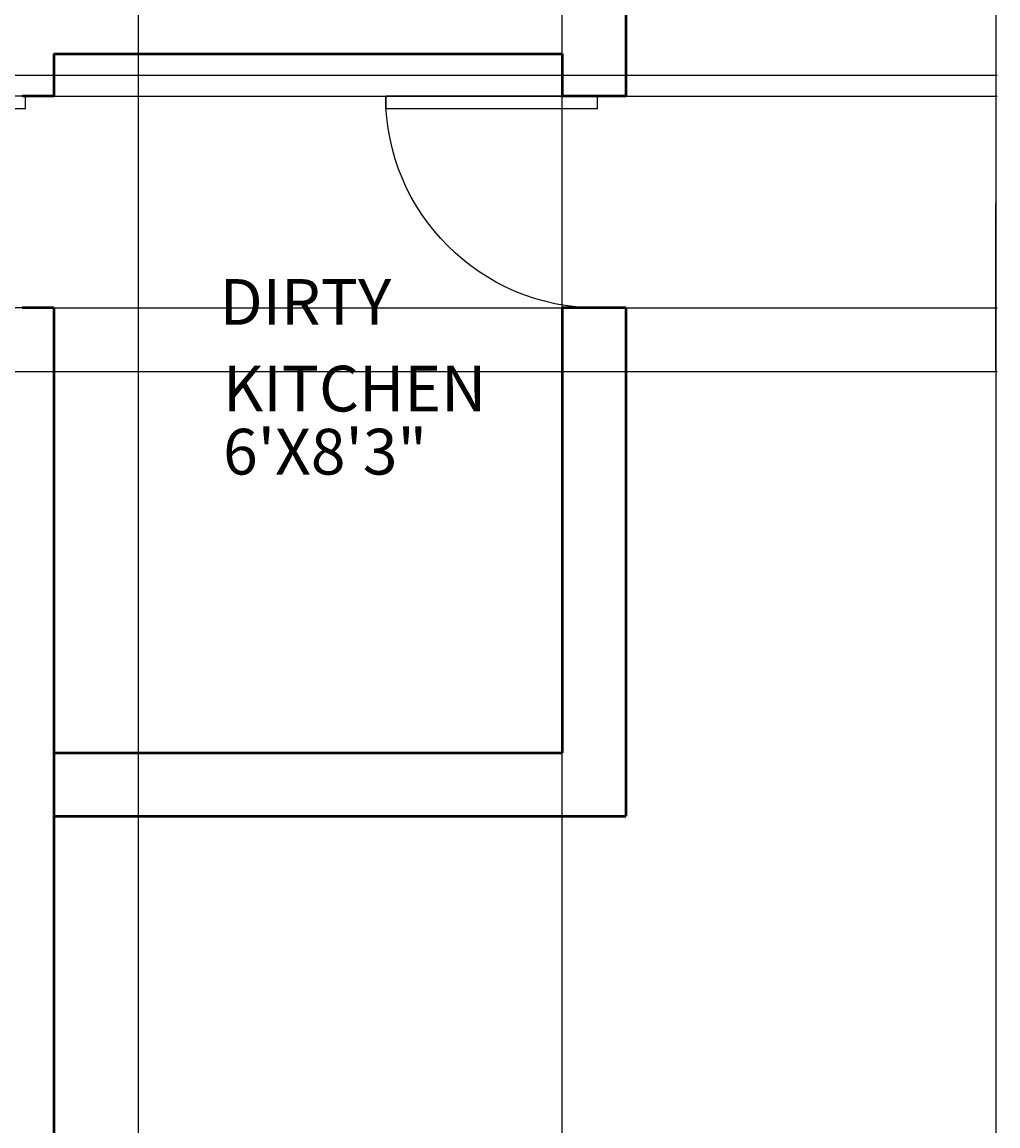
# Model space of a CAD drawing. Units: inches. Extents: x 5375 to 6084, y 16106 to 17259.
# Tile 31 of 32: x 5946 to 6084, y 16776 to 16932. Entities that reach past the tile are written whole.
import ezdxf

# ---------------------------------------------------------------- set-up
doc = ezdxf.new("R2010")
doc.units = ezdxf.units.IN
for name, color, linetype, lineweight in [('A-ANNO-DIMS', 2, 'Continuous', 18), ('A-AREA-IDEN', 5, 'Continuous', 18), ('DOOR', 4, 'Continuous', 25), ('WALL', 6, 'Continuous', 50)]:
    doc.layers.add(name, color=color, linetype=linetype, lineweight=lineweight)
doc.styles.get("Standard").update_dxf_attribs({"font": 'arial.ttf'})
doc.dimstyles.get("Standard").update_dxf_attribs({"dimtxt": 0.18, "dimasz": 0.18, "dimexe": 0.18, "dimexo": 0.0625, "dimgap": 0.09, "dimtad": 0, "dimtih": 1, "dimtoh": 1, "dimdec": 4, "dimzin": 0, "dimdsep": 46, "dimtxsty": 'Standard', "dimcen": 0.09, "dimadec": 0, "dimazin": 0, "dimtfac": 1, "dimtdec": 4, "dimtofl": 0, "dimtmove": 0, "dimatfit": 3, "dimfxl": 1, "dimtolj": 1, "dimtzin": 0, "dimarcsym": 0})

# ---------------------------------------------------------------- blocks, each defined once
blk = doc.blocks.new('*U2')
for p, q in [((0, 0), (0, -100)), ((750, 0), (750, -100))]:
    blk.add_line(p, q)
blk.add_lwpolyline([(0, 0), (0, 750), (43.75, 750), (43.75, 0)], close=True)
blk.add_arc((0, 0), 750, 0, 90)
blk = doc.blocks.new('*D31')
at = {"layer": 'A-ANNO-DIMS', "color": 0, "lineweight": -2, "transparency": 16777216}
for p, q in [((6031.68, 17206.58), (6084.2, 17206.58)), ((6084.02, 17206.4), (6084.02, 16709.66)), ((6084.02, 16212.56), (6084.02, 16709.3)), ((6031.68, 16212.38), (6084.2, 16212.38))]:
    blk.add_line(p, q, dxfattribs=at)
at = {"layer": 'A-ANNO-DIMS', "color": 0, "transparency": 16777216}
for points in [[(6083.99, 17206.4), (6084.05, 17206.4), (6084.02, 17206.58)], [(6083.99, 16212.56), (6084.05, 16212.56), (6084.02, 16212.38)]]:
    blk.add_solid(points, dxfattribs=at)
at = {"layer": 'Defpoints', "color": 0, "transparency": 16777216}
for p in [(6031.62, 17206.58), (6084.02, 17206.58), (6031.62, 16212.38)]:
    blk.add_point(p, dxfattribs=at)
at = {"layer": 'A-ANNO-DIMS', "color": 0, "transparency": 16777216, "insert": (6084.02, 16709.48), "char_height": 0.18, "attachment_point": 5}
blk.add_mtext('\\A1;994.2', dxfattribs=at)
blk = doc.blocks.new('*D41')
at = {"layer": 'A-ANNO-DIMS', "color": 0, "lineweight": -2, "transparency": 16777216}
for p, q in [((5702.18, 16924.58), (6084.2, 16924.58)), ((6084.02, 16924.4), (6084.02, 16903.76)), ((6084.02, 16882.76), (6084.02, 16903.4)), ((5702.18, 16882.58), (6084.2, 16882.58))]:
    blk.add_line(p, q, dxfattribs=at)
at = {"layer": 'A-ANNO-DIMS', "color": 0, "transparency": 16777216}
for points in [[(6083.99, 16924.4), (6084.05, 16924.4), (6084.02, 16924.58)], [(6083.99, 16882.76), (6084.05, 16882.76), (6084.02, 16882.58)]]:
    blk.add_solid(points, dxfattribs=at)
at = {"layer": 'Defpoints', "color": 0, "transparency": 16777216}
for p in [(5702.12, 16924.58), (6084.02, 16924.58), (5702.12, 16882.58)]:
    blk.add_point(p, dxfattribs=at)
at = {"layer": 'A-ANNO-DIMS', "color": 0, "transparency": 16777216, "insert": (6084.02, 16903.58), "char_height": 0.18, "attachment_point": 5}
blk.add_mtext('\\A1;42', dxfattribs=at)
blk = doc.blocks.new('*D45')
at = {"layer": 'A-ANNO-DIMS', "color": 0, "lineweight": -2, "transparency": 16777216}
for p, q in [((5950.68, 16921.58), (6084.2, 16921.58)), ((6084.02, 16921.4), (6084.02, 16906.76)), ((6084.02, 16891.76), (6084.02, 16906.4)), ((5950.68, 16891.58), (6084.2, 16891.58))]:
    blk.add_line(p, q, dxfattribs=at)
at = {"layer": 'A-ANNO-DIMS', "color": 0, "transparency": 16777216}
for points in [[(6083.99, 16921.4), (6084.05, 16921.4), (6084.02, 16921.58)], [(6083.99, 16891.76), (6084.05, 16891.76), (6084.02, 16891.58)]]:
    blk.add_solid(points, dxfattribs=at)
at = {"layer": 'Defpoints', "color": 0, "transparency": 16777216}
for p in [(5950.62, 16921.58), (6084.02, 16921.58), (5950.62, 16891.58)]:
    blk.add_point(p, dxfattribs=at)
at = {"layer": 'A-ANNO-DIMS', "color": 0, "transparency": 16777216, "insert": (6084.02, 16906.58), "char_height": 0.18, "attachment_point": 5}
blk.add_mtext('\\A1;30', dxfattribs=at)
blk = doc.blocks.new('*D48')
at = {"layer": 'A-ANNO-DIMS', "color": 0, "lineweight": -2, "transparency": 16777216}
for p, q in [((5962.62, 16411.64), (5962.62, 17259.16)), ((6022.62, 16411.64), (6022.62, 17259.16)), ((5962.8, 17258.98), (5992.4, 17258.98)), ((6022.44, 17258.98), (5992.84, 17258.98))]:
    blk.add_line(p, q, dxfattribs=at)
at = {"layer": 'A-ANNO-DIMS', "color": 0, "transparency": 16777216}
for points in [[(5962.8, 17259.01), (5962.8, 17258.95), (5962.62, 17258.98)], [(6022.44, 17259.01), (6022.44, 17258.95), (6022.62, 17258.98)]]:
    blk.add_solid(points, dxfattribs=at)
at = {"layer": 'Defpoints', "color": 0, "transparency": 16777216}
for p in [(6022.62, 17258.98), (5962.62, 16411.58), (6022.62, 16411.58)]:
    blk.add_point(p, dxfattribs=at)
at = {"layer": 'A-ANNO-DIMS', "color": 0, "transparency": 16777216, "insert": (5992.62, 17258.98), "char_height": 0.18, "attachment_point": 5}
blk.add_mtext('\\A1;60', dxfattribs=at)

msp = doc.modelspace()

# ---------------------------------------------------------------- linework, layer by layer
at = {"layer": 'WALL'}
for p, q in [((6031.6199, 17206.5793), (6031.6199, 16921.5793)), ((5950.6199, 16927.5793), (5950.6199, 16921.5793)), ((5950.6199, 16927.5793), (6022.6199, 16927.5793)), ((6022.6199, 16927.5793), (6022.6199, 16921.5793)), ((5950.6199, 16921.5793), (5946.1199, 16921.5793)), ((6031.6199, 16921.5793), (6022.6199, 16921.5793)), ((5950.6199, 16891.5793), (5946.1199, 16891.5793)), ((5950.6199, 16891.5793), (5950.6199, 16828.5793)), ((6031.6199, 16891.5793), (6022.6199, 16891.5793)), ((6022.6199, 16891.5793), (6022.6199, 16828.5793)), ((6031.6199, 16891.5793), (6031.6199, 16819.5793)), ((5950.6199, 16828.5793), (6022.6199, 16828.5793)), ((5950.6199, 16828.5793), (5950.6199, 16699.5793)), ((5950.6199, 16819.5793), (6031.6199, 16819.5793))]:
    msp.add_line(p, q, dxfattribs=at)

# ---------------------------------------------------------------- block references
at = {"layer": 'DOOR', "xscale": -0.0399999999999999, "yscale": 0.0399999999999999, "zscale": 0.0399999999999999, "rotation": 90}
for p in [(5946.6199, 16921.5793), (6027.6199, 16921.5793)]:
    msp.add_blockref('*U2', p, dxfattribs=at)

# ---------------------------------------------------------------- texts
at = {"layer": 'A-AREA-IDEN'}
for s, p in [('DIRTY', (5974.1196, 16889.195)), ('KITCHEN', (5974.5889, 16876.9197)), ('6\'X8\'3"', (5974.5889, 16867.9866))]:
    msp.add_text(s, height=6.47981, dxfattribs=at).set_placement(p)

# ---------------------------------------------------------------- dimensions: what is measured, and where the dimension line sits
at = {"layer": 'A-ANNO-DIMS'}
dim = msp.add_linear_dim(base=(6022.6199, 17258.9793), p1=(5962.6199, 16411.5793), p2=(6022.6199, 16411.5793), dimstyle='Standard', override={"dimdec": 0, "dimlfac": 1, "dimrnd": 0, "dimzin": 0, "dimdsep": 46, "dimlunit": 2}, dxfattribs=at)
dim.commit()
dim.dimension.update_dxf_attribs({"geometry": '*D48', "text_midpoint": (5992.6199, 17258.9793)})
for base, p1, p2, override, picture, middle in [((6084.0199, 17206.5793), (6031.6199, 16212.3785), (6031.6199, 17206.5793), {"dimdec": 1, "dimlfac": 1, "dimrnd": 0, "dimzin": 0, "dimdsep": 46, "dimlunit": 2}, '*D31', (6084.0199, 16709.4789)), ((6084.0199, 16924.5793), (5702.1199, 16882.5793), (5702.1199, 16924.5793), {"dimdec": 0, "dimlfac": 1, "dimrnd": 0, "dimzin": 0, "dimdsep": 46, "dimlunit": 2}, '*D41', (6084.0199, 16903.5793)), ((6084.0199, 16921.5793), (5950.6199, 16891.5793), (5950.6199, 16921.5793), {"dimdec": 0, "dimlfac": 1, "dimrnd": 0, "dimzin": 0, "dimdsep": 46, "dimlunit": 2}, '*D45', (6084.0199, 16906.5793))]:
    dim = msp.add_linear_dim(base=base, p1=p1, p2=p2, angle=90, dimstyle='Standard', override=override, dxfattribs=at)
    dim.commit()
    dim.dimension.update_dxf_attribs({"geometry": picture, "text_midpoint": middle})

doc.saveas('drawing.dxf')
